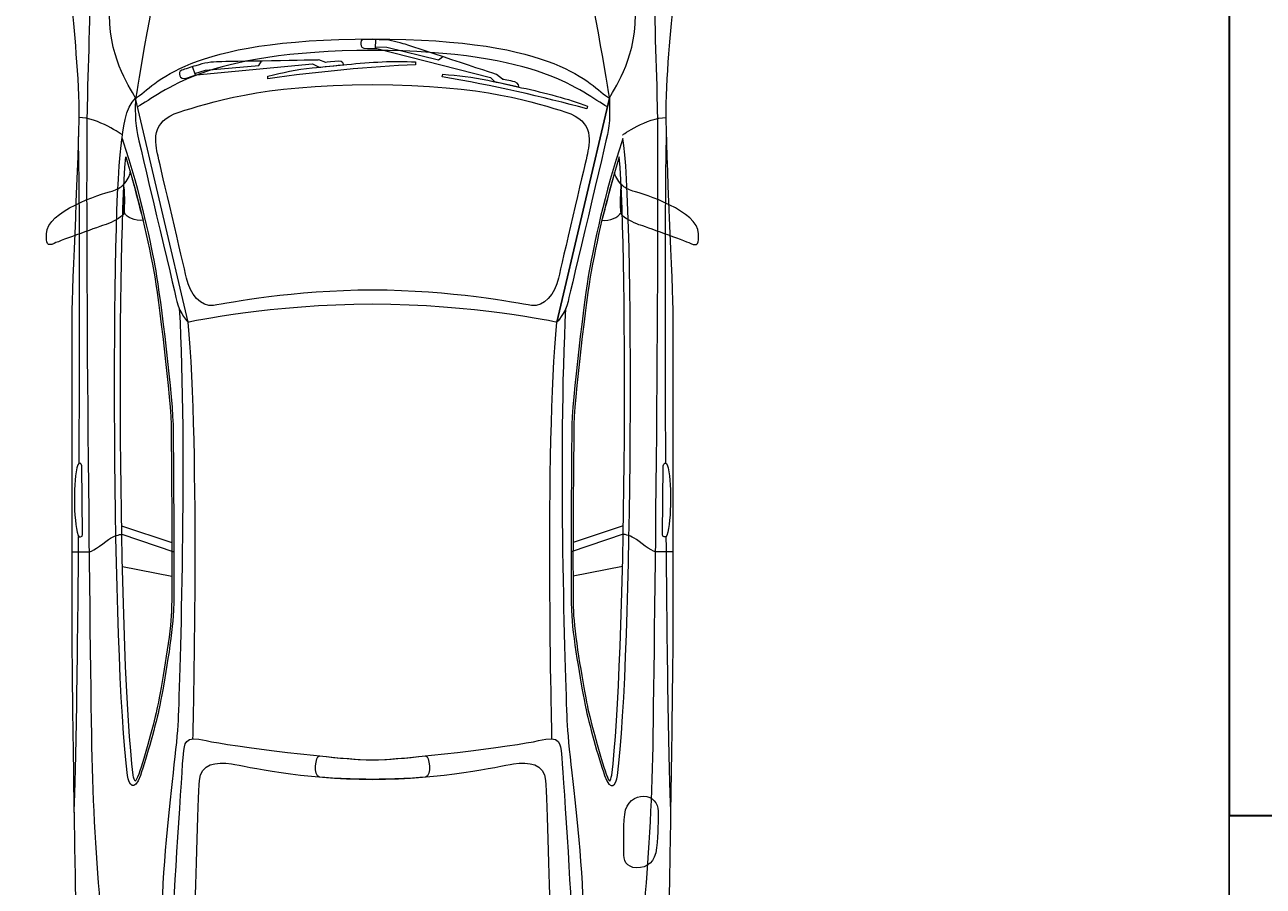
# Model space of a CAD drawing. Units: inches. Extents: x 1911 to 3278, y 2022 to 3108.
# Tile 4 of 13: x 2045 to 2120, y 2178 to 2230. Entities that reach past the tile are written whole.
import ezdxf

# ---------------------------------------------------------------- set-up
doc = ezdxf.new("R2010")
doc.units = ezdxf.units.IN
for name, color, linetype, lineweight in [('A-ANNO-DIMS', 2, 'Continuous', 18), ('A-WALL', 7, 'Continuous', 35), ('AUDI', 7, 'Continuous', 18)]:
    doc.layers.add(name, color=color, linetype=linetype, lineweight=lineweight)
doc.styles.get("Standard").update_dxf_attribs({"font": 'arial.ttf'})
doc.dimstyles.get("Standard").update_dxf_attribs({"dimtxt": 0.18, "dimasz": 0.18, "dimexe": 0.18, "dimexo": 0.0625, "dimgap": 0.09, "dimtad": 0, "dimtih": 1, "dimtoh": 1, "dimdec": 4, "dimzin": 0, "dimdsep": 46, "dimtxsty": 'Standard', "dimcen": 0.09, "dimadec": 0, "dimazin": 0, "dimtfac": 1, "dimtdec": 4, "dimtofl": 0, "dimtmove": 0, "dimatfit": 3, "dimfxl": 1, "dimtolj": 1, "dimtzin": 0, "dimarcsym": 0})

# ---------------------------------------------------------------- blocks, each defined once
blk = doc.blocks.new('*D68')
at = {"layer": 'A-ANNO-DIMS', "color": 0, "lineweight": -2, "transparency": 16777216}
for p, q in [((2016.834, 2263.811), (2016.834, 2048.124)), ((2117.834, 2263.811), (2117.834, 2048.124)), ((2017.014, 2048.304), (2067.071, 2048.304)), ((2117.654, 2048.304), (2067.597, 2048.304))]:
    blk.add_line(p, q, dxfattribs=at)
at = {"layer": 'A-ANNO-DIMS', "color": 0, "transparency": 16777216}
for points in [[(2017.014, 2048.334), (2017.014, 2048.274), (2016.834, 2048.304)], [(2117.654, 2048.334), (2117.654, 2048.274), (2117.834, 2048.304)]]:
    blk.add_solid(points, dxfattribs=at)
at = {"layer": 'Defpoints', "color": 0, "transparency": 16777216}
for p in [(2016.834, 2263.873), (2117.834, 2263.873), (2117.834, 2048.304)]:
    blk.add_point(p, dxfattribs=at)
at = {"layer": 'A-ANNO-DIMS', "color": 0, "transparency": 16777216, "insert": (2067.334, 2048.304), "char_height": 0.18, "attachment_point": 5}
blk.add_mtext('\\A1;101', dxfattribs=at)
blk = doc.blocks.new('*D70')
at = {"layer": 'A-ANNO-DIMS', "color": 0, "lineweight": -2, "transparency": 16777216}
for p, q in [((2134.103, 2181.811), (2134.103, 2048.124)), ((2016.834, 2133.811), (2016.834, 2048.124)), ((2017.014, 2048.304), (2075.014, 2048.304)), ((2133.923, 2048.304), (2075.924, 2048.304))]:
    blk.add_line(p, q, dxfattribs=at)
at = {"layer": 'A-ANNO-DIMS', "color": 0, "transparency": 16777216}
for points in [[(2017.014, 2048.334), (2017.014, 2048.274), (2016.834, 2048.304)], [(2133.923, 2048.334), (2133.923, 2048.274), (2134.103, 2048.304)]]:
    blk.add_solid(points, dxfattribs=at)
at = {"layer": 'Defpoints', "color": 0, "transparency": 16777216}
for p in [(2134.103, 2181.873), (2016.834, 2133.873), (2134.103, 2048.304)]:
    blk.add_point(p, dxfattribs=at)
at = {"layer": 'A-ANNO-DIMS', "color": 0, "transparency": 16777216, "insert": (2075.469, 2048.304), "char_height": 0.18, "attachment_point": 5}
blk.add_mtext('\\A1;117.27', dxfattribs=at)

msp = doc.modelspace()

# ---------------------------------------------------------------- linework, layer by layer
at = {"layer": 'A-WALL'}
for p, q in [((2117.8344, 2263.8733), (2117.8344, 2217.8733)), ((2117.8344, 2217.8733), (2117.8344, 2181.8733)), ((2117.8344, 2181.8733), (2134.1034, 2181.8733))]:
    msp.add_line(p, q, dxfattribs=at)
at = {"layer": 'AUDI'}
for points, knots in [([(2065.7636, 2161.2036), (2052.3657, 2161.35), (2050.4204, 2165.8553), (2049.5983, 2168.8238), (2049.5983, 2168.8238), (2049.0621, 2170.5764), (2048.6333, 2171.9712), (2048.4187, 2172.6866), (2048.4187, 2172.6866), (2048.2042, 2173.4019), (2047.7397, 2175.5836), (2047.7038, 2177.4077), (2047.7038, 2177.4077), (2047.6679, 2179.2318), (2047.491, 2190.1075), (2047.491, 2193.1091), (2047.491, 2193.1091), (2047.491, 2196.1105), (2047.491, 2210.1722), (2047.491, 2212.1725), (2047.491, 2212.1725), (2047.491, 2214.1727), (2047.9184, 2222.1512), (2047.9184, 2224.6905), (2047.9184, 2224.6905), (2047.9184, 2227.23), (2047.491, 2230.416), (2047.491, 2231.7362), (2047.491, 2231.7362), (2047.491, 2233.0566), (2047.7395, 2240.034), (2047.8468, 2241.572), (2047.8468, 2241.572), (2047.9542, 2243.11), (2048.5301, 2243.9822), (2049.0266, 2245.0771), (2049.0266, 2245.0771), (2050.9569, 2249.333), (2055.8898, 2251.6577), (2056.426, 2252.0154), (2056.426, 2252.0154), (2056.9622, 2252.3732), (2057.5315, 2252.5675), (2058.2133, 2252.5675), (2058.2133, 2252.5675), (2058.8952, 2252.5675), (2059.0712, 2252.2302), (2059.3573, 2252.3017), (2059.3573, 2252.3017), (2059.6432, 2252.3732), (2060.3558, 2252.5675), (2061.1448, 2252.5675), (2061.1448, 2252.5675), (2061.9338, 2252.5675), (2065.7636, 2252.5675), (2065.7636, 2252.5675), (2065.7636, 2252.5675), (2065.7636, 2252.5675), (2069.5936, 2252.5675), (2070.3825, 2252.5675), (2070.3825, 2252.5675), (2071.1717, 2252.5675), (2071.8841, 2252.3732), (2072.1701, 2252.3017), (2072.1701, 2252.3017), (2072.4561, 2252.2302), (2072.6322, 2252.5675), (2073.314, 2252.5675), (2073.314, 2252.5675), (2073.9959, 2252.5675), (2074.5651, 2252.3732), (2075.1013, 2252.0154), (2075.1013, 2252.0154), (2075.6375, 2251.6577), (2080.5704, 2249.333), (2082.5007, 2245.0771), (2082.5007, 2245.0771), (2082.9972, 2243.9822), (2083.5731, 2243.1099), (2083.6805, 2241.572), (2083.6805, 2241.572), (2083.7879, 2240.0341), (2084.0364, 2233.0565), (2084.0364, 2231.7362), (2084.0364, 2231.7362), (2084.0364, 2230.4161), (2083.609, 2227.23), (2083.609, 2224.6905), (2083.609, 2224.6905), (2083.609, 2222.1512), (2084.0364, 2214.1727), (2084.0364, 2212.1725), (2084.0364, 2212.1725), (2084.0364, 2210.1722), (2084.0364, 2196.1105), (2084.0364, 2193.1091), (2084.0364, 2193.1091), (2084.0364, 2190.1075), (2083.8594, 2179.2318), (2083.8235, 2177.4077), (2083.8235, 2177.4077), (2083.7877, 2175.5836), (2083.3232, 2173.4019), (2083.1086, 2172.6866), (2083.1086, 2172.6866), (2082.8941, 2171.9712), (2082.4652, 2170.5764), (2081.9291, 2168.8238), (2081.9291, 2168.8238), (2081.107, 2165.8553), (2079.1616, 2161.35), (2065.7636, 2161.2036)], [0, 0, 0, 0, 0.0357143, 0.0357143, 0.0357143, 0.0357143, 0.0714286, 0.0714286, 0.0714286, 0.0714286, 0.1071429, 0.1071429, 0.1071429, 0.1071429, 0.1428571, 0.1428571, 0.1428571, 0.1428572, 0.1785714, 0.1785714, 0.1785714, 0.1785714, 0.2142857, 0.2142857, 0.2142857, 0.2142857, 0.25, 0.25, 0.25, 0.25, 0.2857143, 0.2857143, 0.2857143, 0.2857143, 0.3214286, 0.3214286, 0.3214286, 0.3214286, 0.3571429, 0.3571429, 0.3571429, 0.3571429, 0.3928571, 0.3928571, 0.3928571, 0.3928572, 0.4285714, 0.4285714, 0.4285714, 0.4285714, 0.4642857, 0.4642857, 0.4642857, 0.4642857, 0.5, 0.5, 0.5, 0.5, 0.5357143, 0.5357143, 0.5357143, 0.5357143, 0.5714286, 0.5714286, 0.5714286, 0.5714286, 0.6071429, 0.6071429, 0.6071429, 0.6071429, 0.6428571, 0.6428571, 0.6428571, 0.6428572, 0.6785714, 0.6785714, 0.6785714, 0.6785714, 0.7142857, 0.7142857, 0.7142857, 0.7142857, 0.75, 0.75, 0.75, 0.75, 0.7857143, 0.7857143, 0.7857143, 0.7857143, 0.8214286, 0.8214286, 0.8214286, 0.8214286, 0.8571429, 0.8571429, 0.8571429, 0.8571429, 0.8928571, 0.8928571, 0.8928571, 0.8928572, 0.9285714, 0.9285714, 0.9285714, 0.9285714, 0.9642857, 0.9642857, 0.9642857, 0.9642857, 1, 1, 1, 1]), ([(2051.3626, 2225.4871), (2050.9454, 2226.322), (2049.6509, 2227.988), (2049.7888, 2231.1364), (2049.7888, 2231.1364), (2049.9267, 2234.2849), (2050.4858, 2242.9716), (2050.9873, 2245.7351)], [0, 0, 0, 0, 0.5, 0.5, 0.5, 0.5, 1, 1, 1, 1]), ([(2080.1647, 2225.4871), (2080.582, 2226.322), (2081.8765, 2227.988), (2081.7386, 2231.1364), (2081.7386, 2231.1364), (2081.6006, 2234.2849), (2081.0416, 2242.9716), (2080.54, 2245.7351)], [0, 0, 0, 0, 0.5, 0.5, 0.5, 0.5, 1, 1, 1, 1]), ([(2050.2266, 2168.7846), (2049.5535, 2172.1525), (2048.8368, 2178.9728), (2048.7144, 2186.0758), (2048.7144, 2186.0758), (2048.5919, 2193.1787), (2048.2861, 2220.4882), (2048.4696, 2226.2439), (2048.4696, 2226.2439), (2048.6532, 2231.9997), (2048.7559, 2239.2607), (2049.7755, 2244.2027)], [0, 0, 0, 0, 0.3333333, 0.3333333, 0.3333333, 0.3333333, 0.6666667, 0.6666667, 0.6666667, 0.6666667, 1, 1, 1, 1]), ([(2081.3007, 2168.7846), (2081.9739, 2172.1525), (2082.6906, 2178.9728), (2082.813, 2186.0758), (2082.813, 2186.0758), (2082.9355, 2193.1787), (2083.2413, 2220.4882), (2083.0577, 2226.2439), (2083.0577, 2226.2439), (2082.8742, 2231.9997), (2082.7714, 2239.2607), (2081.7518, 2244.2027)], [0, 0, 0, 0, 0.3333333, 0.3333333, 0.3333333, 0.3333333, 0.6666667, 0.6666667, 0.6666667, 0.6666667, 1, 1, 1, 1]), ([(2065.7636, 2212.9638), (2071.8282, 2212.9638), (2076.9669, 2211.8667), (2076.9669, 2211.8667), (2076.9669, 2211.8667), (2076.9669, 2211.8667), (2080.1647, 2225.4871), (2080.1647, 2225.4871), (2080.1647, 2225.4871), (2078.8855, 2226.3099), (2077.2188, 2229.0981), (2065.7636, 2229.0981), (2065.7636, 2229.0981), (2054.3085, 2229.0981), (2052.6418, 2226.3099), (2051.3626, 2225.4871), (2051.3626, 2225.4871), (2051.3626, 2225.4871), (2054.5605, 2211.8667), (2054.5605, 2211.8667), (2054.5605, 2211.8667), (2054.5605, 2211.8667), (2059.6991, 2212.9637), (2065.7636, 2212.9638)], [0, 0, 0, 0, 0.1666667, 0.1666667, 0.1666667, 0.1666667, 0.3333333, 0.3333333, 0.3333333, 0.3333333, 0.5, 0.5, 0.5, 0.5, 0.6666667, 0.6666667, 0.6666667, 0.6666667, 0.8333333, 0.8333333, 0.8333333, 0.8333333, 1, 1, 1, 1]), ([(2065.7636, 2212.9638), (2071.8282, 2212.9638), (2076.9669, 2211.8667), (2076.9669, 2211.8667), (2076.9669, 2211.8667), (2076.9669, 2211.8667), (2080.1647, 2225.4871), (2080.1647, 2225.4871), (2080.1647, 2225.4871), (2078.8855, 2226.3099), (2077.2188, 2229.0981), (2065.7636, 2229.0981), (2065.7636, 2229.0981), (2054.3085, 2229.0981), (2052.6418, 2226.3099), (2051.3626, 2225.4871), (2051.3626, 2225.4871), (2051.3626, 2225.4871), (2054.5605, 2211.8667), (2054.5605, 2211.8667), (2054.5605, 2211.8667), (2054.5605, 2211.8667), (2059.6991, 2212.9638), (2065.7636, 2212.9638)], [0, 0, 0, 0, 0.1666667, 0.1666667, 0.1666667, 0.1666667, 0.3333333, 0.3333333, 0.3333333, 0.3333333, 0.5, 0.5, 0.5, 0.5, 0.6666667, 0.6666667, 0.6666667, 0.6666667, 0.8333333, 0.8333333, 0.8333333, 0.8333333, 1, 1, 1, 1]), ([(2066.1787, 2229.0507), (2066.7344, 2229.0507), (2067.1399, 2228.9604), (2067.6207, 2228.8101), (2067.6207, 2228.8101), (2067.9811, 2228.705), (2073.2981, 2226.9315), (2073.2981, 2226.9315), (2073.2981, 2226.9315), (2073.2981, 2226.9315), (2073.6587, 2226.646), (2073.6587, 2226.646), (2073.6587, 2226.646), (2073.6587, 2226.646), (2074.1393, 2226.5558), (2074.4097, 2226.4959), (2074.4097, 2226.4959), (2074.6802, 2226.4208), (2074.6501, 2226.1801), (2074.6501, 2226.1801), (2074.6501, 2226.1801), (2074.6501, 2226.1801), (2073.1779, 2226.5108), (2073.1779, 2226.5108), (2073.1779, 2226.5108), (2073.1779, 2226.5108), (2072.9377, 2226.7515), (2072.9377, 2226.7515), (2072.9377, 2226.7515), (2072.9377, 2226.7515), (2066.0283, 2228.5096), (2066.0283, 2228.5096), (2066.0283, 2228.5096), (2066.0283, 2228.5096), (2065.803, 2228.5096), (2065.4575, 2228.5096), (2065.4575, 2228.5096), (2065.1119, 2228.5245), (2065.0521, 2228.6449), (2065.0521, 2228.7799), (2065.0521, 2228.7799), (2065.0521, 2228.9303), (2065.0672, 2229.0658), (2065.2774, 2229.0658), (2065.2774, 2229.0658), (2065.4876, 2229.0807), (2065.8331, 2229.0658), (2066.1787, 2229.0507)], [0, 0, 0, 0, 0.0833333, 0.0833333, 0.0833333, 0.0833333, 0.1666667, 0.1666667, 0.1666667, 0.1666667, 0.25, 0.25, 0.25, 0.25, 0.3333333, 0.3333333, 0.3333333, 0.3333333, 0.4166667, 0.4166667, 0.4166667, 0.4166667, 0.5, 0.5, 0.5, 0.5, 0.5833333, 0.5833333, 0.5833333, 0.5833333, 0.6666667, 0.6666667, 0.6666667, 0.6666667, 0.75, 0.75, 0.75, 0.75, 0.8333333, 0.8333333, 0.8333333, 0.8333333, 0.9166667, 0.9166667, 0.9166667, 0.9166667, 1, 1, 1, 1]), ([(2080.0439, 2224.9729), (2078.4865, 2225.801), (2076.0796, 2228.3951), (2065.7636, 2228.3951), (2065.7636, 2228.3951), (2055.4478, 2228.3951), (2053.0409, 2225.801), (2051.4834, 2224.9728)], [0, 0, 0, 0, 0.5, 0.5, 0.5, 0.5, 1, 1, 1, 1]), ([(2065.9534, 2228.6148), (2065.9534, 2228.6148), (2066.6442, 2228.5997), (2066.6442, 2228.5997), (2066.6442, 2228.5997), (2066.6442, 2228.5997), (2069.7683, 2227.8181), (2069.7683, 2227.8181), (2069.7683, 2227.8181), (2069.7683, 2227.8181), (2070.0238, 2228.0135), (2070.0238, 2228.0135)], [0, 0, 0, 0, 0.3333333, 0.3333333, 0.3333333, 0.3333333, 0.6666667, 0.6666667, 0.6666667, 0.6666667, 1, 1, 1, 1]), ([(2055.0333, 2227.4724), (2055.5441, 2227.653), (2055.9646, 2227.6979), (2056.4754, 2227.713), (2056.4754, 2227.713), (2056.8508, 2227.7131), (2062.4985, 2227.8181), (2062.4985, 2227.8181), (2062.4985, 2227.8181), (2062.4985, 2227.8181), (2062.9341, 2227.6678), (2062.9341, 2227.6678), (2062.9341, 2227.6678), (2062.9341, 2227.6678), (2063.4297, 2227.7281), (2063.7001, 2227.7432), (2063.7001, 2227.7432), (2063.9707, 2227.7731), (2064.0155, 2227.5327), (2064.0155, 2227.5327), (2064.0155, 2227.5327), (2064.0155, 2227.5327), (2062.5287, 2227.3824), (2062.5287, 2227.3824), (2062.5287, 2227.3824), (2062.5287, 2227.3824), (2062.1231, 2227.5778), (2062.1231, 2227.5778), (2062.1231, 2227.5778), (2062.1231, 2227.5778), (2055.0635, 2226.9164), (2055.0635, 2226.9164), (2055.0635, 2226.9164), (2055.0635, 2226.9164), (2054.8533, 2226.8415), (2054.5228, 2226.7363), (2054.5228, 2226.7363), (2054.2072, 2226.6311), (2054.1021, 2226.7212), (2054.0571, 2226.8565), (2054.0571, 2226.8565), (2054.0118, 2227.0065), (2053.9819, 2227.1273), (2054.1773, 2227.2021), (2054.1773, 2227.2021), (2054.3724, 2227.2622), (2054.7029, 2227.3673), (2055.0333, 2227.4724)], [0, 0, 0, 0, 0.0833333, 0.0833333, 0.0833333, 0.0833333, 0.1666667, 0.1666667, 0.1666667, 0.1666667, 0.25, 0.25, 0.25, 0.25, 0.3333333, 0.3333333, 0.3333333, 0.3333333, 0.4166667, 0.4166667, 0.4166667, 0.4166667, 0.5, 0.5, 0.5, 0.5, 0.5833333, 0.5833333, 0.5833333, 0.5833333, 0.6666667, 0.6666667, 0.6666667, 0.6666667, 0.75, 0.75, 0.75, 0.75, 0.8333333, 0.8333333, 0.8333333, 0.8333333, 0.9166667, 0.9166667, 0.9166667, 0.9166667, 1, 1, 1, 1]), ([(2055.0333, 2227.4724), (2055.5441, 2227.653), (2055.9646, 2227.6979), (2056.4754, 2227.713), (2056.4754, 2227.713), (2056.8508, 2227.713), (2062.4985, 2227.8181), (2062.4985, 2227.8181), (2062.4985, 2227.8181), (2062.4985, 2227.8181), (2062.9341, 2227.6678), (2062.9341, 2227.6678), (2062.9341, 2227.6678), (2062.9341, 2227.6678), (2063.4297, 2227.7281), (2063.7001, 2227.7432), (2063.7001, 2227.7432), (2063.9707, 2227.7731), (2064.0155, 2227.5327), (2064.0155, 2227.5327), (2064.0155, 2227.5327), (2064.0155, 2227.5327), (2062.5287, 2227.3824), (2062.5287, 2227.3824), (2062.5287, 2227.3824), (2062.5287, 2227.3824), (2062.1231, 2227.5778), (2062.1231, 2227.5778), (2062.1231, 2227.5778), (2062.1231, 2227.5778), (2055.0635, 2226.9164), (2055.0635, 2226.9164), (2055.0635, 2226.9164), (2055.0635, 2226.9164), (2054.8533, 2226.8415), (2054.5228, 2226.7363), (2054.5228, 2226.7363), (2054.2072, 2226.6311), (2054.1021, 2226.7212), (2054.0571, 2226.8565), (2054.0571, 2226.8565), (2054.0118, 2227.0065), (2053.9819, 2227.1273), (2054.1773, 2227.2021), (2054.1773, 2227.2021), (2054.3724, 2227.2622), (2054.7029, 2227.3673), (2055.0333, 2227.4724)], [0, 0, 0, 0, 0.0833333, 0.0833333, 0.0833333, 0.0833333, 0.1666667, 0.1666667, 0.1666667, 0.1666667, 0.25, 0.25, 0.25, 0.25, 0.3333333, 0.3333333, 0.3333333, 0.3333333, 0.4166667, 0.4166667, 0.4166667, 0.4166667, 0.5, 0.5, 0.5, 0.5, 0.5833333, 0.5833333, 0.5833333, 0.5833333, 0.6666667, 0.6666667, 0.6666667, 0.6666667, 0.75, 0.75, 0.75, 0.75, 0.8333333, 0.8333333, 0.8333333, 0.8333333, 0.9166667, 0.9166667, 0.9166667, 0.9166667, 1, 1, 1, 1]), ([(2054.9734, 2226.9917), (2054.9734, 2226.9917), (2055.6191, 2227.2021), (2055.6191, 2227.2021), (2055.6191, 2227.2021), (2055.6191, 2227.2021), (2058.8486, 2227.4875), (2058.8486, 2227.4875), (2058.8486, 2227.4875), (2058.8486, 2227.4875), (2059.0288, 2227.7432), (2059.0288, 2227.7432)], [0, 0, 0, 0, 0.3333333, 0.3333333, 0.3333333, 0.3333333, 0.6666667, 0.6666667, 0.6666667, 0.6666667, 1, 1, 1, 1]), ([(2068.3716, 2227.698), (2067.0798, 2227.788), (2065.6677, 2227.6828), (2064.2107, 2227.5478), (2064.2107, 2227.5478), (2063.505, 2227.4724), (2062.7988, 2227.4125), (2062.108, 2227.3371), (2062.108, 2227.3371), (2061.1317, 2227.2471), (2060.3056, 2227.0517), (2059.4043, 2226.8415), (2059.4043, 2226.8415), (2059.4043, 2226.8415), (2059.4043, 2226.6759), (2059.4043, 2226.6759), (2059.4043, 2226.6759), (2062.4684, 2227.1121), (2065.6528, 2227.4125), (2068.3867, 2227.5327), (2068.3867, 2227.5327), (2068.3867, 2227.5327), (2068.3716, 2227.698), (2068.3716, 2227.698)], [0, 0, 0, 0, 0.1666667, 0.1666667, 0.1666667, 0.1666667, 0.3333333, 0.3333333, 0.3333333, 0.3333333, 0.5, 0.5, 0.5, 0.5, 0.6666667, 0.6666667, 0.6666667, 0.6666667, 0.8333333, 0.8333333, 0.8333333, 0.8333333, 1, 1, 1, 1]), ([(2078.8408, 2225.008), (2077.6391, 2225.4737), (2076.2721, 2225.8194), (2074.8302, 2226.1349), (2074.8302, 2226.1349), (2074.1393, 2226.2853), (2073.4485, 2226.4505), (2072.7725, 2226.5858), (2072.7725, 2226.5858), (2071.8262, 2226.7967), (2070.9699, 2226.8714), (2070.0389, 2226.9466), (2070.0389, 2226.9466), (2070.0389, 2226.9466), (2069.9937, 2226.7967), (2069.9937, 2226.7967), (2069.9937, 2226.7967), (2073.0429, 2226.2703), (2076.1522, 2225.579), (2078.7957, 2224.8427), (2078.7957, 2224.8427), (2078.7957, 2224.8427), (2078.8408, 2225.008), (2078.8408, 2225.008)], [0, 0, 0, 0, 0.1666667, 0.1666667, 0.1666667, 0.1666667, 0.3333333, 0.3333333, 0.3333333, 0.3333333, 0.5, 0.5, 0.5, 0.5, 0.6666667, 0.6666667, 0.6666667, 0.6666667, 0.8333333, 0.8333333, 0.8333333, 0.8333333, 1, 1, 1, 1]), ([(2065.7636, 2213.8208), (2070.5775, 2213.8208), (2074.5177, 2213.0314), (2075.4297, 2212.8935), (2075.4297, 2212.8935), (2076.1739, 2212.7808), (2076.8621, 2213.5859), (2077.0708, 2214.5514), (2077.0708, 2214.5514), (2077.2793, 2215.5167), (2078.6093, 2221.1523), (2078.7919, 2221.9612), (2078.7919, 2221.9612), (2078.9744, 2222.77), (2079.2873, 2224.1007), (2077.5141, 2224.6485), (2077.5141, 2224.6485), (2075.7408, 2225.1966), (2072.6063, 2226.3183), (2065.7636, 2226.3183), (2065.7636, 2226.3183), (2058.9211, 2226.3183), (2055.7865, 2225.1965), (2054.0133, 2224.6485), (2054.0133, 2224.6485), (2052.24, 2224.1008), (2052.553, 2222.77), (2052.7355, 2221.9612), (2052.7355, 2221.9612), (2052.918, 2221.1524), (2054.248, 2215.5167), (2054.4566, 2214.5514), (2054.4566, 2214.5514), (2054.6652, 2213.586), (2055.3534, 2212.7808), (2056.0976, 2212.8935), (2056.0976, 2212.8935), (2057.0097, 2213.0314), (2060.9498, 2213.8208), (2065.7636, 2213.8208)], [0, 0, 0, 0, 0.1, 0.1, 0.1, 0.1, 0.2, 0.2, 0.2, 0.2, 0.3, 0.3, 0.3, 0.3, 0.4, 0.4, 0.4, 0.4, 0.5, 0.5, 0.5, 0.5, 0.6, 0.6, 0.6, 0.6, 0.7, 0.7, 0.7, 0.7, 0.8, 0.8, 0.8, 0.8, 0.9, 0.9, 0.9, 0.9, 1, 1, 1, 1]), ([(2051.3626, 2225.4871), (2051.3626, 2225.4871), (2054.5605, 2211.8667), (2054.5605, 2211.8667), (2054.5605, 2211.8667), (2054.5605, 2211.8667), (2054.0606, 2212.3621), (2053.8778, 2213.1392), (2053.8778, 2213.1392), (2053.695, 2213.9162), (2051.5738, 2222.794), (2051.4367, 2223.5252), (2051.4367, 2223.5252), (2051.2996, 2224.2564), (2051.3626, 2225.4871), (2051.3626, 2225.4871)], [0, 0, 0, 0, 0.25, 0.25, 0.25, 0.25, 0.5, 0.5, 0.5, 0.5, 0.75, 0.75, 0.75, 0.75, 1, 1, 1, 1]), ([(2051.3626, 2225.4871), (2051.3626, 2225.4871), (2054.5605, 2211.8667), (2054.5605, 2211.8667), (2054.5605, 2211.8667), (2054.5605, 2211.8667), (2054.0606, 2212.3621), (2053.8778, 2213.1392), (2053.8778, 2213.1392), (2053.695, 2213.9162), (2051.5738, 2222.794), (2051.4367, 2223.5252), (2051.4367, 2223.5252), (2051.2996, 2224.2564), (2051.3626, 2225.4871), (2051.3626, 2225.4871)], [0, 0, 0, 0, 0.25, 0.25, 0.25, 0.25, 0.5, 0.5, 0.5, 0.5, 0.75, 0.75, 0.75, 0.75, 1, 1, 1, 1]), ([(2080.1647, 2225.4871), (2080.1647, 2225.4871), (2076.9669, 2211.8667), (2076.9669, 2211.8667), (2076.9669, 2211.8667), (2076.9669, 2211.8667), (2077.4668, 2212.3621), (2077.6495, 2213.1392), (2077.6495, 2213.1392), (2077.8323, 2213.9162), (2079.9535, 2222.794), (2080.0906, 2223.5252), (2080.0906, 2223.5252), (2080.2277, 2224.2564), (2080.1647, 2225.4871), (2080.1647, 2225.4871)], [0, 0, 0, 0, 0.25, 0.25, 0.25, 0.25, 0.5, 0.5, 0.5, 0.5, 0.75, 0.75, 0.75, 0.75, 1, 1, 1, 1]), ([(2050.8698, 2184.3067), (2050.9411, 2183.7465), (2051.2876, 2183.2388), (2051.6588, 2184.3067), (2051.6588, 2184.3067), (2052.03, 2185.3746), (2052.6333, 2187.5568), (2052.8188, 2188.4853), (2052.8188, 2188.4853), (2053.0044, 2189.4137), (2053.5614, 2192.4778), (2053.6541, 2194.01), (2053.6541, 2194.01), (2053.7468, 2195.5421), (2053.6541, 2203.3883), (2053.6541, 2205.2453), (2053.6541, 2205.2453), (2053.6541, 2207.1025), (2052.8653, 2213.4631), (2052.5868, 2214.9951), (2052.5868, 2214.9951), (2052.3083, 2216.5272), (2051.7051, 2219.5914), (2050.5434, 2223.0429), (2050.5434, 2223.0429), (2049.8491, 2219.2201), (2049.9416, 2191.5958), (2050.8698, 2184.3067)], [0, 0, 0, 0, 0.1428571, 0.1428571, 0.1428571, 0.1428572, 0.2857143, 0.2857143, 0.2857143, 0.2857143, 0.4285714, 0.4285714, 0.4285714, 0.4285714, 0.5714286, 0.5714286, 0.5714286, 0.5714286, 0.7142857, 0.7142857, 0.7142857, 0.7142857, 0.8571429, 0.8571429, 0.8571429, 0.8571429, 1, 1, 1, 1]), ([(2080.6576, 2184.3067), (2080.5863, 2183.7465), (2080.2397, 2183.2388), (2079.8685, 2184.3067), (2079.8685, 2184.3067), (2079.4973, 2185.3746), (2078.8942, 2187.5568), (2078.7085, 2188.4853), (2078.7085, 2188.4853), (2078.523, 2189.4137), (2077.9659, 2192.4778), (2077.8732, 2194.01), (2077.8732, 2194.01), (2077.7805, 2195.5421), (2077.8732, 2203.3883), (2077.8732, 2205.2453), (2077.8732, 2205.2453), (2077.8732, 2207.1025), (2078.6621, 2213.4631), (2078.9406, 2214.9951), (2078.9406, 2214.9951), (2079.219, 2216.5272), (2079.8223, 2219.5914), (2080.9839, 2223.0429), (2080.9839, 2223.0429), (2081.6783, 2219.2201), (2081.5858, 2191.5958), (2080.6576, 2184.3067)], [0, 0, 0, 0, 0.1428571, 0.1428571, 0.1428571, 0.1428572, 0.2857143, 0.2857143, 0.2857143, 0.2857143, 0.4285714, 0.4285714, 0.4285714, 0.4285714, 0.5714286, 0.5714286, 0.5714286, 0.5714286, 0.7142857, 0.7142857, 0.7142857, 0.7142857, 0.8571429, 0.8571429, 0.8571429, 0.8571429, 1, 1, 1, 1]), ([(2051.2226, 2184.3366), (2051.2226, 2184.3366), (2051.2226, 2184.3366), (2051.2226, 2184.3366), (2051.2226, 2184.3366), (2051.2487, 2184.1314), (2051.3045, 2184.0123), (2051.3451, 2183.955), (2051.3451, 2183.955), (2051.3875, 2184.0055), (2051.4606, 2184.1171), (2051.5535, 2184.3845), (2051.5535, 2184.3845), (2051.9153, 2185.4252), (2052.5179, 2187.5957), (2052.7049, 2188.5316), (2052.7049, 2188.5316), (2052.9291, 2189.6527), (2053.4496, 2192.5921), (2053.5361, 2194.0242), (2053.5361, 2194.0242), (2053.604, 2195.1446), (2053.5714, 2199.7231), (2053.55, 2202.7528), (2053.55, 2202.7528), (2053.55, 2202.7528), (2053.5357, 2205.2453), (2053.5357, 2205.2453), (2053.5357, 2205.2453), (2053.5357, 2207.0972), (2052.7383, 2213.4883), (2052.4723, 2214.9527), (2052.4723, 2214.9527), (2052.0271, 2217.4016), (2051.4498, 2219.7334), (2050.7669, 2221.9202), (2050.7669, 2221.9202), (2050.2213, 2215.5853), (2050.3625, 2191.0904), (2051.2226, 2184.3366)], [0, 0, 0, 0, 0.1, 0.1, 0.1, 0.1, 0.2, 0.2, 0.2, 0.2, 0.3, 0.3, 0.3, 0.3, 0.4, 0.4, 0.4, 0.4, 0.5, 0.5, 0.5, 0.5, 0.6, 0.6, 0.6, 0.6, 0.7, 0.7, 0.7, 0.7, 0.8, 0.8, 0.8, 0.8, 0.9, 0.9, 0.9, 0.9, 1, 1, 1, 1]), ([(2080.3047, 2184.3366), (2080.3047, 2184.3366), (2080.3047, 2184.3366), (2080.3047, 2184.3366), (2080.3047, 2184.3366), (2080.2786, 2184.1314), (2080.2228, 2184.0123), (2080.1823, 2183.955), (2080.1823, 2183.955), (2080.1399, 2184.0055), (2080.0668, 2184.1171), (2079.9739, 2184.3845), (2079.9739, 2184.3845), (2079.6121, 2185.4252), (2079.0094, 2187.5957), (2078.8224, 2188.5316), (2078.8224, 2188.5316), (2078.5983, 2189.6527), (2078.0778, 2192.5921), (2077.9912, 2194.0242), (2077.9912, 2194.0242), (2077.9233, 2195.1446), (2077.956, 2199.7231), (2077.9773, 2202.7528), (2077.9773, 2202.7528), (2077.9773, 2202.7528), (2077.9916, 2205.2453), (2077.9916, 2205.2453), (2077.9916, 2205.2453), (2077.9916, 2207.0972), (2078.789, 2213.4883), (2079.0551, 2214.9527), (2079.0551, 2214.9527), (2079.5002, 2217.4016), (2080.0776, 2219.7334), (2080.7605, 2221.9202), (2080.7605, 2221.9202), (2081.3061, 2215.5853), (2081.1648, 2191.0904), (2080.3047, 2184.3366)], [0, 0, 0, 0, 0.1, 0.1, 0.1, 0.1, 0.2, 0.2, 0.2, 0.2, 0.3, 0.3, 0.3, 0.3, 0.4, 0.4, 0.4, 0.4, 0.5, 0.5, 0.5, 0.5, 0.6, 0.6, 0.6, 0.6, 0.7, 0.7, 0.7, 0.7, 0.8, 0.8, 0.8, 0.8, 0.9, 0.9, 0.9, 0.9, 1, 1, 1, 1]), ([(2050.6208, 2220.2328), (2050.6946, 2219.851), (2050.7013, 2219.0195), (2050.6567, 2218.4472), (2050.6567, 2218.4472), (2050.6732, 2218.4654), (2050.6915, 2218.484), (2050.7027, 2218.5002), (2050.7027, 2218.5002), (2050.8054, 2218.2822), (2051.3339, 2217.9946), (2051.8197, 2218.0743), (2051.8197, 2218.0743), (2051.756, 2218.3408), (2051.0462, 2220.9973), (2051.0462, 2220.9973), (2051.0462, 2220.9973), (2051.0173, 2220.7775), (2050.8789, 2220.4791), (2050.6208, 2220.2328)], [0, 0, 0, 0, 0.2, 0.2, 0.2, 0.2, 0.4, 0.4, 0.4, 0.4, 0.6, 0.6, 0.6, 0.6, 0.8, 0.8, 0.8, 0.8, 1, 1, 1, 1]), ([(2080.9065, 2220.2328), (2080.8328, 2219.851), (2080.8261, 2219.0195), (2080.8707, 2218.4472), (2080.8707, 2218.4472), (2080.8542, 2218.4654), (2080.8359, 2218.484), (2080.8246, 2218.5002), (2080.8246, 2218.5002), (2080.722, 2218.2822), (2080.1935, 2217.9946), (2079.7076, 2218.0743), (2079.7076, 2218.0743), (2079.7714, 2218.3408), (2080.4812, 2220.9973), (2080.4812, 2220.9973), (2080.4812, 2220.9973), (2080.5101, 2220.7775), (2080.6484, 2220.4791), (2080.9065, 2220.2328)], [0, 0, 0, 0, 0.2, 0.2, 0.2, 0.2, 0.4, 0.4, 0.4, 0.4, 0.6, 0.6, 0.6, 0.6, 0.8, 0.8, 0.8, 0.8, 1, 1, 1, 1]), ([(2050.6208, 2220.2328), (2050.4476, 2220.0674), (2050.2219, 2219.9249), (2049.9334, 2219.8475), (2049.9334, 2219.8475), (2049.2153, 2219.6548), (2045.9842, 2218.6416), (2045.9457, 2217.2559), (2045.9457, 2217.2559), (2045.9457, 2216.6657), (2045.9583, 2216.4605), (2046.42, 2216.6657), (2046.42, 2216.6657), (2046.8816, 2216.871), (2049.2027, 2217.7047), (2049.5873, 2217.8202), (2049.5873, 2217.8202), (2049.9414, 2217.9268), (2050.4649, 2218.238), (2050.6567, 2218.4472), (2050.6567, 2218.4472), (2050.7013, 2219.0195), (2050.6946, 2219.851), (2050.6208, 2220.2328)], [0, 0, 0, 0, 0.1666667, 0.1666667, 0.1666667, 0.1666667, 0.3333333, 0.3333333, 0.3333333, 0.3333333, 0.5, 0.5, 0.5, 0.5, 0.6666667, 0.6666667, 0.6666667, 0.6666667, 0.8333333, 0.8333333, 0.8333333, 0.8333333, 1, 1, 1, 1]), ([(2080.9065, 2220.2328), (2081.0797, 2220.0674), (2081.3054, 2219.9249), (2081.5939, 2219.8475), (2081.5939, 2219.8475), (2082.312, 2219.6548), (2085.5432, 2218.6416), (2085.5817, 2217.2559), (2085.5817, 2217.2559), (2085.5817, 2216.6657), (2085.569, 2216.4605), (2085.1074, 2216.6657), (2085.1074, 2216.6657), (2084.6457, 2216.871), (2082.3247, 2217.7047), (2081.94, 2217.8202), (2081.94, 2217.8202), (2081.5859, 2217.9268), (2081.0624, 2218.238), (2080.8707, 2218.4472), (2080.8707, 2218.4472), (2080.8261, 2219.0195), (2080.8328, 2219.851), (2080.9065, 2220.2328)], [0, 0, 0, 0, 0.1666667, 0.1666667, 0.1666667, 0.1666667, 0.3333333, 0.3333333, 0.3333333, 0.3333333, 0.5, 0.5, 0.5, 0.5, 0.6666667, 0.6666667, 0.6666667, 0.6666667, 0.8333333, 0.8333333, 0.8333333, 0.8333333, 1, 1, 1, 1]), ([(2054.0235, 2212.6996), (2054.5037, 2204.0341), (2054.0518, 2190.4068), (2053.9475, 2187.6412), (2053.9475, 2187.6412), (2053.8432, 2184.8757), (2052.1504, 2175.4823), (2053.3909, 2169.197)], [0, 0, 0, 0, 0.5, 0.5, 0.5, 0.5, 1, 1, 1, 1]), ([(2077.5039, 2212.6996), (2077.0237, 2204.0341), (2077.4756, 2190.4068), (2077.5799, 2187.6412), (2077.5799, 2187.6412), (2077.6842, 2184.8757), (2079.3769, 2175.4823), (2078.1365, 2169.197)], [0, 0, 0, 0, 0.5, 0.5, 0.5, 0.5, 1, 1, 1, 1]), ([(2048.1457, 2198.9684), (2048.1457, 2198.8047), (2047.9218, 2198.7432), (2047.8721, 2198.907), (2047.8721, 2198.907), (2047.7226, 2199.378), (2047.6484, 2200.2172), (2047.6484, 2201.0567), (2047.6484, 2201.0567), (2047.6484, 2201.8961), (2047.6979, 2202.7149), (2047.8471, 2203.2063), (2047.8471, 2203.2063), (2047.8967, 2203.3496), (2048.0956, 2203.3086), (2048.0956, 2203.1448), (2048.0956, 2203.1448), (2048.0956, 2203.1448), (2048.1457, 2198.9684), (2048.1457, 2198.9684)], [0, 0, 0, 0, 0.2, 0.2, 0.2, 0.2, 0.4, 0.4, 0.4, 0.4, 0.6, 0.6, 0.6, 0.6, 0.8, 0.8, 0.8, 0.8, 1, 1, 1, 1]), ([(2083.3816, 2198.9684), (2083.3816, 2198.8047), (2083.6055, 2198.7432), (2083.6552, 2198.907), (2083.6552, 2198.907), (2083.8048, 2199.378), (2083.8789, 2200.2172), (2083.8789, 2201.0567), (2083.8789, 2201.0567), (2083.8789, 2201.8961), (2083.8294, 2202.7149), (2083.6803, 2203.2063), (2083.6803, 2203.2063), (2083.6306, 2203.3496), (2083.4317, 2203.3086), (2083.4317, 2203.1448), (2083.4317, 2203.1448), (2083.4317, 2203.1448), (2083.3816, 2198.9684), (2083.3816, 2198.9684)], [0, 0, 0, 0, 0.2, 0.2, 0.2, 0.2, 0.4, 0.4, 0.4, 0.4, 0.6, 0.6, 0.6, 0.6, 0.8, 0.8, 0.8, 0.8, 1, 1, 1, 1]), ([(2047.491, 2197.917), (2047.491, 2197.917), (2048.2961, 2197.9169), (2048.5605, 2197.9169), (2048.5605, 2197.9169), (2048.8249, 2197.9169), (2049.5258, 2198.5582), (2049.8491, 2198.7456), (2049.8491, 2198.7456), (2050.1724, 2198.933), (2050.5275, 2198.9775), (2050.5275, 2198.9775)], [0, 0, 0, 0, 0.3333333, 0.3333333, 0.3333333, 0.3333333, 0.6666667, 0.6666667, 0.6666667, 0.6666667, 1, 1, 1, 1]), ([(2084.0364, 2197.917), (2084.0364, 2197.917), (2083.2313, 2197.9169), (2082.9668, 2197.9169), (2082.9668, 2197.9169), (2082.7024, 2197.9169), (2082.0016, 2198.5582), (2081.6783, 2198.7456), (2081.6783, 2198.7456), (2081.355, 2198.933), (2080.9999, 2198.9775), (2080.9999, 2198.9775)], [0, 0, 0, 0, 0.3333333, 0.3333333, 0.3333333, 0.3333333, 0.6666667, 0.6666667, 0.6666667, 0.6666667, 1, 1, 1, 1]), ([(2065.7636, 2170.8144), (2070.2681, 2170.8144), (2074.0546, 2171.7187), (2075.793, 2172.345), (2075.793, 2172.345), (2077.5314, 2172.9711), (2077.8792, 2174.5714), (2077.8792, 2175.3715), (2077.8792, 2175.3715), (2077.8792, 2176.1716), (2077.3227, 2184.9729), (2077.2533, 2185.5992), (2077.2533, 2185.5992), (2077.1838, 2186.2254), (2077.2184, 2186.782), (2075.8625, 2186.434), (2075.8625, 2186.434), (2074.5064, 2186.0861), (2067.4483, 2185.2513), (2065.7636, 2185.2513), (2065.7636, 2185.2513), (2064.0791, 2185.2513), (2057.0209, 2186.0861), (2055.6649, 2186.434), (2055.6649, 2186.434), (2054.3089, 2186.782), (2054.3435, 2186.2254), (2054.274, 2185.5992), (2054.274, 2185.5992), (2054.2046, 2184.9729), (2053.6482, 2176.1716), (2053.6482, 2175.3715), (2053.6482, 2175.3715), (2053.6482, 2174.5714), (2053.996, 2172.9711), (2055.7344, 2172.345), (2055.7344, 2172.345), (2057.4727, 2171.7187), (2061.2592, 2170.8144), (2065.7636, 2170.8144)], [0, 0, 0, 0, 0.1, 0.1, 0.1, 0.1, 0.2, 0.2, 0.2, 0.2, 0.3, 0.3, 0.3, 0.3, 0.4, 0.4, 0.4, 0.4, 0.5, 0.5, 0.5, 0.5, 0.6, 0.6, 0.6, 0.6, 0.7, 0.7, 0.7, 0.7, 0.8, 0.8, 0.8, 0.8, 0.9, 0.9, 0.9, 0.9, 1, 1, 1, 1]), ([(2065.7636, 2170.8144), (2070.2681, 2170.8144), (2074.0546, 2171.7187), (2075.793, 2172.345), (2075.793, 2172.345), (2077.5314, 2172.9711), (2077.8792, 2174.5714), (2077.8792, 2175.3715), (2077.8792, 2175.3715), (2077.8792, 2176.1716), (2077.3227, 2184.9729), (2077.2533, 2185.5992), (2077.2533, 2185.5992), (2077.1838, 2186.2254), (2077.2184, 2186.782), (2075.8625, 2186.434), (2075.8625, 2186.434), (2074.5064, 2186.0861), (2067.4483, 2185.2513), (2065.7636, 2185.2513), (2065.7636, 2185.2513), (2064.0791, 2185.2513), (2057.0209, 2186.0861), (2055.6649, 2186.434), (2055.6649, 2186.434), (2054.3089, 2186.782), (2054.3435, 2186.2254), (2054.274, 2185.5992), (2054.274, 2185.5992), (2054.2046, 2184.9729), (2053.6482, 2176.1716), (2053.6482, 2175.3715), (2053.6482, 2175.3715), (2053.6482, 2174.5714), (2053.996, 2172.9711), (2055.7344, 2172.345), (2055.7344, 2172.345), (2057.4727, 2171.7187), (2061.2592, 2170.8144), (2065.7636, 2170.8144)], [0, 0, 0, 0, 0.1, 0.1, 0.1, 0.1, 0.2, 0.2, 0.2, 0.2, 0.3, 0.3, 0.3, 0.3, 0.4, 0.4, 0.4, 0.4, 0.5, 0.5, 0.5, 0.5, 0.6, 0.6, 0.6, 0.6, 0.7, 0.7, 0.7, 0.7, 0.8, 0.8, 0.8, 0.8, 0.9, 0.9, 0.9, 0.9, 1, 1, 1, 1]), ([(2065.7636, 2171.8557), (2067.9003, 2171.8557), (2074.6107, 2172.7972), (2075.3757, 2173.2147), (2075.3757, 2173.2147), (2076.1407, 2173.6321), (2076.5579, 2174.2235), (2076.5579, 2175.3715), (2076.5579, 2175.3715), (2076.5579, 2176.5194), (2076.3491, 2182.9553), (2076.2797, 2183.9989), (2076.2797, 2183.9989), (2076.2102, 2185.0426), (2075.2715, 2185.147), (2074.3327, 2185.0078), (2074.3327, 2185.0078), (2073.3938, 2184.8686), (2070.0908, 2184.0686), (2065.7636, 2184.0686), (2065.7636, 2184.0686), (2061.4365, 2184.0686), (2058.1335, 2184.8686), (2057.1947, 2185.0078), (2057.1947, 2185.0078), (2056.2559, 2185.147), (2055.3171, 2185.0426), (2055.2476, 2183.9989), (2055.2476, 2183.9989), (2055.1782, 2182.9553), (2054.9693, 2176.5194), (2054.9693, 2175.3715), (2054.9693, 2175.3715), (2054.9693, 2174.2235), (2055.3866, 2173.6321), (2056.1516, 2173.2147), (2056.1516, 2173.2147), (2056.9166, 2172.7973), (2063.627, 2171.8557), (2065.7636, 2171.8557)], [0, 0, 0, 0, 0.1, 0.1, 0.1, 0.1, 0.2, 0.2, 0.2, 0.2, 0.3, 0.3, 0.3, 0.3, 0.4, 0.4, 0.4, 0.4, 0.5, 0.5, 0.5, 0.5, 0.6, 0.6, 0.6, 0.6, 0.7, 0.7, 0.7, 0.7, 0.8, 0.8, 0.8, 0.8, 0.9, 0.9, 0.9, 0.9, 1, 1, 1, 1]), ([(2065.7636, 2184.0686), (2065.7636, 2184.0686), (2068.3149, 2184.1134), (2068.9803, 2184.2115), (2068.9803, 2184.2115), (2069.3965, 2184.2729), (2069.2008, 2185.5176), (2069.0062, 2185.4988), (2069.0062, 2185.4988), (2067.7836, 2185.3801), (2066.7556, 2185.2513), (2065.7636, 2185.2513), (2065.7636, 2185.2513), (2064.7717, 2185.2513), (2063.7437, 2185.3801), (2062.5212, 2185.4988), (2062.5212, 2185.4988), (2062.3266, 2185.5176), (2062.1308, 2184.2729), (2062.547, 2184.2115), (2062.547, 2184.2115), (2063.2124, 2184.1134), (2065.7636, 2184.0686), (2065.7636, 2184.0686)], [0, 0, 0, 0, 0.1666667, 0.1666667, 0.1666667, 0.1666667, 0.3333333, 0.3333333, 0.3333333, 0.3333333, 0.5, 0.5, 0.5, 0.5, 0.6666667, 0.6666667, 0.6666667, 0.6666667, 0.8333333, 0.8333333, 0.8333333, 0.8333333, 1, 1, 1, 1]), ([(2081.0471, 2179.6345), (2080.9988, 2179.1799), (2081.1616, 2178.7086), (2081.8212, 2178.696), (2081.8212, 2178.696), (2082.481, 2178.6833), (2082.9341, 2179.0347), (2083.0308, 2179.906), (2083.0308, 2179.906), (2083.1275, 2180.7773), (2083.1275, 2181.6485), (2083.1275, 2182.1327), (2083.1275, 2182.1327), (2083.1275, 2182.6167), (2082.7888, 2183.0523), (2082.2567, 2183.0523), (2082.2567, 2183.0523), (2081.7245, 2183.0523), (2081.1924, 2182.7136), (2081.0956, 2181.9391), (2081.0956, 2181.9391), (2080.9988, 2181.1645), (2081.0471, 2179.6345), (2081.0471, 2179.6345)], [0, 0, 0, 0, 0.1666667, 0.1666667, 0.1666667, 0.1666667, 0.3333333, 0.3333333, 0.3333333, 0.3333333, 0.5, 0.5, 0.5, 0.5, 0.6666667, 0.6666667, 0.6666667, 0.6666667, 0.8333333, 0.8333333, 0.8333333, 0.8333333, 1, 1, 1, 1])]:
    msp.add_open_spline(points, degree=3, knots=knots, dxfattribs=at)
for points in [[(2056.3231, 2250.1984), (2055.1434, 2246.4433), (2051.5649, 2227.2055), (2051.3563, 2225.3269)], [(2075.2042, 2250.1984), (2076.384, 2246.4433), (2079.9624, 2227.2055), (2080.1711, 2225.3269)], [(2065.9534, 2228.5096), (2065.9534, 2228.5096), (2065.9682, 2229.0658), (2065.9682, 2229.0658)], [(2055.0034, 2226.8865), (2055.0034, 2226.8865), (2054.8229, 2227.4125), (2054.8229, 2227.4125)], [(2050.5189, 2222.8221), (2050.5884, 2223.4484), (2050.7363, 2225.0063), (2051.3626, 2225.4871)], [(2050.5688, 2223.2596), (2050.5688, 2223.2596), (2049.068, 2224.3177), (2047.9159, 2224.3177)], [(2080.9585, 2223.2596), (2080.9585, 2223.2596), (2082.4594, 2224.3177), (2083.6115, 2224.3177)], [(2047.9345, 2203.2889), (2047.9803, 2211.5888), (2047.975, 2219.8422), (2047.8909, 2223.1652)], [(2083.5929, 2203.2889), (2083.5471, 2211.5888), (2083.5524, 2219.8422), (2083.6365, 2223.1652)], [(2054.8539, 2186.5352), (2054.8539, 2186.5352), (2055.299, 2204.2856), (2054.5605, 2211.8667)], [(2076.6735, 2186.5352), (2076.6735, 2186.5352), (2076.2283, 2204.2856), (2076.9669, 2211.8667)], [(2050.5185, 2199.4833), (2050.5185, 2199.4833), (2053.5746, 2198.4799), (2053.5746, 2198.4799)], [(2081.0088, 2199.4833), (2081.0088, 2199.4833), (2077.9527, 2198.4799), (2077.9527, 2198.4799)], [(2047.6258, 2182.0661), (2047.7446, 2184.1853), (2047.8454, 2191.1479), (2047.9051, 2198.8488)], [(2050.5275, 2198.9775), (2050.5275, 2198.9775), (2053.6944, 2197.917), (2053.6944, 2197.917)], [(2080.9999, 2198.9775), (2080.9999, 2198.9775), (2077.8329, 2197.917), (2077.8329, 2197.917)], [(2083.9015, 2182.0661), (2083.7828, 2184.1853), (2083.6819, 2191.1479), (2083.6222, 2198.8488)], [(2050.5678, 2197.0251), (2050.5678, 2197.0251), (2053.5759, 2196.4239), (2053.5759, 2196.4239)], [(2080.9595, 2197.0251), (2080.9595, 2197.0251), (2077.9515, 2196.4239), (2077.9515, 2196.4239)]]:
    msp.add_open_spline(points, degree=3, dxfattribs=at)

# ---------------------------------------------------------------- dimensions: what is measured, and where the dimension line sits
at = {"layer": 'A-ANNO-DIMS'}
for base, p1, p2, override, picture, middle in [((2117.8344, 2048.3043), (2016.8344, 2263.8733), (2117.8344, 2263.8733), {"dimdec": 0, "dimlfac": 1, "dimrnd": 0, "dimzin": 0, "dimdsep": 46, "dimlunit": 2}, '*D68', (2067.3344, 2048.3043)), ((2134.1034, 2048.3043), (2016.8344, 2133.8733), (2134.1034, 2181.8733), {"dimdec": 2, "dimlfac": 1, "dimrnd": 0, "dimzin": 0, "dimdsep": 46, "dimlunit": 2}, '*D70', (2075.4689, 2048.3043))]:
    dim = msp.add_linear_dim(base=base, p1=p1, p2=p2, dimstyle='Standard', override=override, dxfattribs=at)
    dim.commit()
    dim.dimension.update_dxf_attribs({"geometry": picture, "text_midpoint": middle})

doc.saveas('drawing.dxf')
